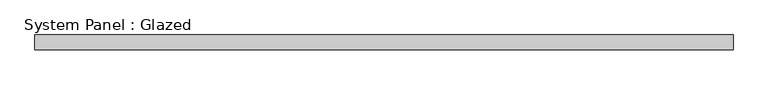
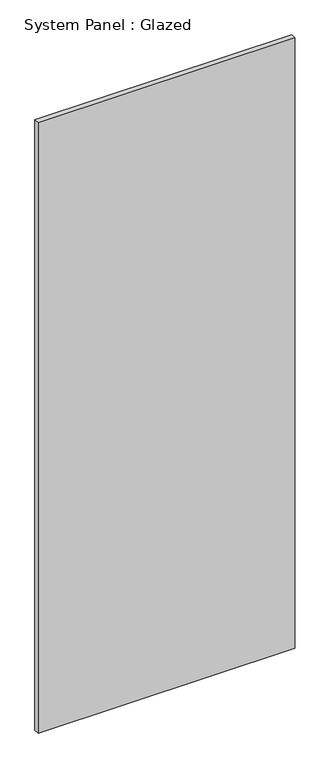
"""IFC4 building model written with IfcOpenShell, lengths in millimetres: plate geometry, System Panel : Glazed."""

from ifc_helpers import new_model, si_unit, origin, origin_with_axes, place, context, project, spatial, polyline, outline, extrude, source, transform, mapped, element, save


def system_panel_glazed_00f127ae(model_context):
    return source(origin(), model_context, "Body", "SweptSolid", [
        extrude(outline(polyline([(596.9, 24.5), (-596.9, 24.5), (-596.9, 49.5), (596.9, 49.5), (596.9, 24.5)])), origin_with_axes(), (0.0, 0.0, 1.0), 3000.0),
    ])


if __name__ == "__main__":
    model = new_model("IFC4")
    model_context = context("Model", 3, world=origin())
    ifc_project = project(units=[si_unit("LENGTHUNIT", "METRE", prefix="MILLI")], contexts=[model_context])
    site = spatial("IfcSite", under=ifc_project)
    building = spatial("IfcBuilding", under=site)
    placement = place(None, origin())
    system_panel_glazed_shape = system_panel_glazed_00f127ae(model_context)
    element("IfcPlate", 1, ObjectType="System Panel : Glazed", at=placement, inside=building, context=model_context, shape_type="MappedRepresentation", body=[
        mapped(system_panel_glazed_shape, transform((0.0, 0.0, 0.0), x_axis=(1.0, 0.0, 0.0), y_axis=(0.0, 1.0, 0.0), z_axis=(0.0, 0.0, 1.0))),
    ])
    save(model, "model.ifc")

# Revit data of these elements
# Type "System Panel : Glazed"
#   Keynote = "H11"
#   Construction Type Id = "GSP4R"
#   Analytic Construction = "1/8 in Pilkington single glazing"
#   Visual Light Transmittance = 0.9
#   Solar Heat Gain Coefficient = 0.86
#   Heat Transfer Coefficient (U) = 6.7069 W/(m²·K)
#   Define Thermal Properties by = 1
# Element 1 (IfcPlate, "System Panel : Glazed")
#   Materials on its faces: "Glass"
# Materials
#   "Glass": class "Glass", colour RGB 0 128 192, transparency 0.9, Description = "Soda Lime Glass", Cost = 0
